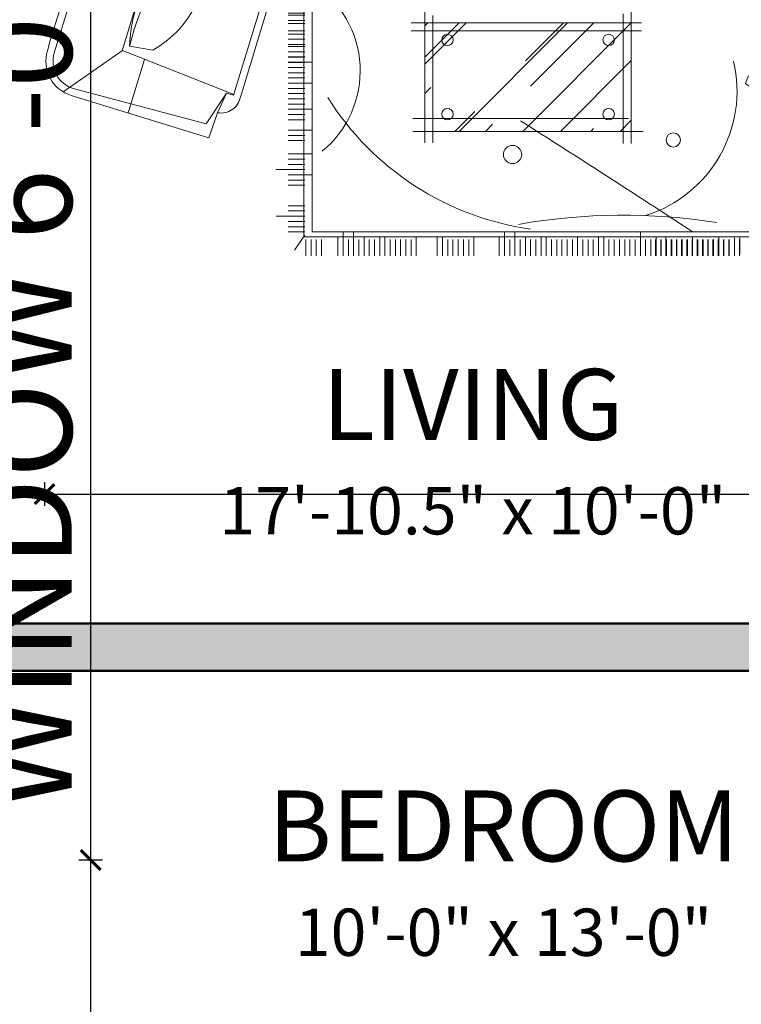
# Model space of a CAD drawing. Units: inches. Extents: x 375 to 1122, y 27 to 1069.
# Tile 73 of 155: x 509 to 601, y 667 to 792. Entities that reach past the tile are written whole.
import ezdxf

# ---------------------------------------------------------------- set-up
doc = ezdxf.new("R2010")
doc.units = ezdxf.units.IN
for name, color, linetype, lineweight in [('A-ANNO-DIMS', 2, 'Continuous', 18), ('A-AREA-IDEN', 7, 'Continuous', 18), ('A-WALL-PATT', 252, 'Continuous', 13), ('Furniture', 30, 'Continuous', 18), ('Walls', 250, 'Continuous', 50)]:
    doc.layers.add(name, color=color, linetype=linetype, lineweight=lineweight)
doc.styles.get("Standard").update_dxf_attribs({"font": 'arial.ttf'})
doc.dimstyles.new('ISO-25', dxfattribs={"dimtxt": 12, "dimasz": 2.5, "dimexe": 1.5, "dimexo": 1.5, "dimtad": 1, "dimdec": 1, "dimlunit": 3, "dimtxsty": 'Standard', "dimblk": 'ARCHTICK', "dimcen": 2.5, "dimadec": 0, "dimazin": 0, "dimtfac": 1, "dimtdec": 1, "dimtmove": 0, "dimatfit": 3, "dimfxl": 1.5, "dimfxlon": 1, "dimarcsym": 0})

# ---------------------------------------------------------------- blocks, each defined once
blk = doc.blocks.new('A$C4DC51D13')
for p, q in [((3265.3, 2996.2), (1188.4, 2996.2)), ((1895.2, 2134), (1895.2, 2996.2)), ((2559.6, 2996.2), (2559.6, 2617.8)), ((277.4, 2939.6), (277.4, 2141.8)), ((943, 2103.5), (943, 2936.7)), ((1188.4, 2962.7), (1862.1, 2962.7)), ((1862.1, 2134), (1862.1, 2962.7)), ((1928.3, 2961.6), (2524.2, 2961.6)), ((1928.3, 2134), (1928.3, 2961.6)), ((2524.2, 2961.6), (2524.2, 2658.6)), ((2590.4, 2962.7), (2590.4, 2654.5)), ((3265.3, 2962.7), (2590.4, 2962.7)), ((1018.2, 2892.3), (232.2, 2892.3)), ((3778.5, 2897), (3631.2, 2747.3)), ((4008.9, 2375.5), (3778.5, 2897)), ((4156.2, 2525.2), (3778.5, 2897)), ((304, 2865.7), (304, 2253.3)), ((916.4, 2865.7), (304, 2865.7)), ((916.4, 2253.3), (916.4, 2865.7)), ((1290.4, 2664.8), (1028, 2870.9)), ((3163.3, 2664.8), (3425.7, 2870.9)), ((1022.9, 2163.8), (1022.9, 2830.3)), ((1056, 2830.3), (1081, 2194.8)), ((3397.7, 2830.3), (3364.5, 2194.8)), ((3430.8, 2163.8), (3430.8, 2830.3)), ((4008.9, 2375.5), (3631.2, 2747.3)), ((423.7, 2370.8), (776.6, 2723.7)), ((427.4, 2727.4), (772.8, 2367.1)), ((497.9, 2644), (497.9, 2699.1)), ((502.2, 2648.3), (502.2, 2701.8)), ((506.4, 2652.2), (506.4, 2704.4)), ((510.6, 2655.8), (510.6, 2706.9)), ((514.9, 2659.2), (514.9, 2709.2)), ((519.1, 2662.3), (519.1, 2711.3)), ((523.3, 2665.1), (523.3, 2713.4)), ((527.5, 2667.8), (527.5, 2715.2)), ((531.8, 2670.2), (531.8, 2717)), ((536, 2672.5), (536, 2718.7)), ((540.2, 2674.6), (540.2, 2720.2)), ((544.4, 2676.5), (544.4, 2721.6)), ((548.7, 2678.2), (548.7, 2722.9)), ((650.1, 2678.8), (650.1, 2723.3)), ((654.3, 2677.1), (654.3, 2722)), ((658.6, 2675.2), (658.6, 2720.7)), ((662.8, 2673.2), (662.8, 2719.2)), ((667, 2671), (667, 2717.6)), ((668.5, 2670.2), (668.5, 2717)), ((671.2, 2668.6), (671.2, 2715.9)), ((672.7, 2667.8), (672.7, 2715.2)), ((675.5, 2666.1), (675.5, 2714)), ((676.9, 2665.1), (676.9, 2713.4)), ((679.7, 2663.3), (679.7, 2712)), ((681.1, 2662.3), (681.1, 2711.3)), ((683.9, 2660.3), (683.9, 2709.9)), ((685.4, 2659.2), (685.4, 2709.2)), ((688.1, 2657), (688.1, 2707.7)), ((689.6, 2655.8), (689.6, 2706.9)), ((692.4, 2653.5), (692.4, 2705.3)), ((693.8, 2652.2), (693.8, 2704.4)), ((696.6, 2649.6), (696.6, 2702.7)), ((698, 2648.3), (698, 2701.8)), ((700.8, 2645.5), (700.8, 2700)), ((702.3, 2644), (702.3, 2699.1)), ((451.5, 2440.6), (451.5, 2654)), ((451.9, 2654.6), (509.2, 2654.6)), ((455.1, 2658.8), (514.4, 2658.8)), ((455.7, 2434.9), (455.7, 2659.6)), ((458.4, 2663.1), (520.2, 2663.1)), ((459.9, 2558.8), (459.9, 2664.9)), ((462, 2667.3), (526.7, 2667.3)), ((464.1, 2583.3), (464.1, 2669.7)), ((465.8, 2671.5), (534.1, 2671.5)), ((468.4, 2596.6), (468.4, 2674.3)), ((469.8, 2675.7), (542.8, 2675.7)), ((472.6, 2606.7), (472.6, 2678.5)), ((476.8, 2615), (476.8, 2682.5)), ((481, 2622.2), (481, 2686.2)), ((485.3, 2628.5), (485.3, 2689.7)), ((489.5, 2634.2), (489.5, 2693)), ((489.5, 2667.3), (489.5, 2633.5)), ((493.7, 2639.3), (493.7, 2696.1)), ((657.4, 2675.7), (730.4, 2675.7)), ((734.5, 2671.5), (666.1, 2671.5)), ((666.1, 2671.5), (734.5, 2671.5)), ((738.2, 2667.3), (673.5, 2667.3)), ((673.5, 2667.3), (738.2, 2667.3)), ((741.8, 2663.1), (680, 2663.1)), ((680, 2663.1), (741.8, 2663.1)), ((745.2, 2658.8), (685.8, 2658.8)), ((685.8, 2658.8), (745.2, 2658.8)), ((748.3, 2654.6), (691, 2654.6)), ((691, 2654.6), (748.3, 2654.6)), ((705, 2641), (705, 2697.2)), ((706.5, 2639.3), (706.5, 2696.1)), ((709.3, 2636), (709.3, 2694.1)), ((710.7, 2634.2), (710.7, 2693)), ((713.5, 2630.5), (713.5, 2690.9)), ((714.9, 2628.5), (714.9, 2689.7)), ((717.7, 2624.4), (717.7, 2687.4)), ((719.2, 2622.2), (719.2, 2686.2)), ((722, 2617.6), (722, 2683.8)), ((723.4, 2615), (723.4, 2682.5)), ((726.2, 2609.7), (726.2, 2679.9)), ((727.6, 2606.7), (727.6, 2678.5)), ((730.4, 2600.3), (730.4, 2675.7)), ((731.9, 2596.6), (731.9, 2674.3)), ((734.6, 2588.4), (734.6, 2671.3)), ((736.1, 2583.3), (736.1, 2669.7)), ((738.9, 2570.4), (738.9, 2666.6)), ((740.3, 2558.8), (740.3, 2664.9)), ((743.1, 2433.1), (743.1, 2661.5)), ((744.5, 2434.9), (744.5, 2659.6)), ((747.3, 2438.6), (747.3, 2656)), ((748.8, 2440.6), (748.8, 2654)), ((1283.3, 2574.2), (1290.4, 2664.8)), ((1290.4, 2664.8), (1894.7, 2664.8)), ((1895.2, 2663.7), (2557.3, 2663.7)), ((2603.6, 2664.8), (2559, 2664.8)), ((3163.3, 2664.8), (2764.7, 2664.8)), ((3170.4, 2574.2), (3163.3, 2664.8)), ((3631.7, 2676.6), (3938.2, 2375)), ((429.1, 2612.3), (475.4, 2612.3)), ((430.3, 2479), (430.3, 2615.5)), ((430.7, 2616.6), (477.7, 2616.6)), ((432.5, 2620.8), (480.2, 2620.8)), ((434.5, 2469.3), (434.5, 2625.2)), ((434.5, 2625), (482.9, 2625)), ((436.5, 2629.2), (485.8, 2629.2)), ((438.7, 2633.5), (488.9, 2633.5)), ((438.8, 2460.9), (438.8, 2633.6)), ((441, 2637.7), (492.3, 2637.7)), ((443, 2453.4), (443, 2641.1)), ((443.5, 2641.9), (496, 2641.9)), ((446.1, 2646.1), (500, 2646.1)), ((447.2, 2446.7), (447.2, 2647.8)), ((448.9, 2650.4), (504.4, 2650.4)), ((751.3, 2650.4), (695.8, 2650.4)), ((695.8, 2650.4), (751.3, 2650.4)), ((754.1, 2646.1), (700.2, 2646.1)), ((700.2, 2646.1), (754.1, 2646.1)), ((756.7, 2641.9), (704.2, 2641.9)), ((704.2, 2641.9), (756.7, 2641.9)), ((759.2, 2637.7), (707.9, 2637.7)), ((707.9, 2637.7), (759.2, 2637.7)), ((761.5, 2633.5), (711.3, 2633.5)), ((711.3, 2633.5), (761.5, 2633.5)), ((763.7, 2629.2), (714.4, 2629.2)), ((714.4, 2629.2), (763.7, 2629.2)), ((765.8, 2625), (717.3, 2625)), ((767.7, 2620.8), (720, 2620.8)), ((769.5, 2616.6), (722.5, 2616.6)), ((771.1, 2612.3), (724.8, 2612.3)), ((751.5, 2444.5), (751.5, 2650)), ((753, 2446.7), (753, 2647.8)), ((755.8, 2451.1), (755.8, 2643.5)), ((757.2, 2453.4), (757.2, 2641.1)), ((760, 2458.3), (760, 2636.3)), ((761.4, 2460.9), (761.4, 2633.6)), ((764.2, 2466.3), (764.2, 2628.2)), ((765.7, 2469.3), (765.7, 2625.2)), ((1798, 2530.2), (1812.1, 2637.9)), ((418.1, 2565.8), (460.7, 2565.8)), ((418.5, 2570.1), (461.3, 2570.1)), ((419.1, 2574.3), (462.1, 2574.3)), ((419.8, 2578.5), (462.9, 2578.5)), ((420.6, 2582.7), (464, 2582.7)), ((421.5, 2587), (465.2, 2587)), ((422.5, 2591.2), (466.5, 2591.2)), ((423.6, 2595.4), (467.9, 2595.4)), ((424.8, 2599.7), (469.6, 2599.7)), ((426.1, 2603.9), (471.3, 2603.9)), ((426.1, 2490.7), (426.1, 2603.9)), ((427.5, 2608.1), (473.3, 2608.1)), ((772.7, 2608.1), (726.9, 2608.1)), ((774.1, 2603.9), (728.9, 2603.9)), ((775.4, 2599.7), (730.7, 2599.7)), ((776.6, 2595.4), (732.3, 2595.4)), ((777.7, 2591.2), (733.7, 2591.2)), ((778.7, 2587), (735.1, 2587)), ((779.6, 2582.7), (736.2, 2582.7)), ((780.4, 2578.5), (737.3, 2578.5)), ((781.1, 2574.3), (738.2, 2574.3)), ((781.7, 2570.1), (738.9, 2570.1)), ((782.2, 2565.8), (739.6, 2565.8)), ((1895.5, 2582.2), (1932.3, 2494.6)), ((417.1, 2548.9), (459.4, 2548.9)), ((417.1, 2544.7), (459.5, 2544.7)), ((417.2, 2553.2), (459.6, 2553.2)), ((417.2, 2540.5), (459.6, 2540.5)), ((417.4, 2557.4), (459.8, 2557.4)), ((417.5, 2536.3), (459.9, 2536.3)), ((417.7, 2561.6), (460.2, 2561.6)), ((417.8, 2532), (460.3, 2532)), ((418.2, 2527.8), (460.8, 2527.8)), ((418.7, 2523.6), (461.4, 2523.6)), ((459.9, 2429.7), (459.9, 2535.7)), ((781.6, 2523.6), (738.8, 2523.6)), ((782.1, 2527.8), (739.4, 2527.8)), ((782.5, 2532), (740, 2532)), ((782.5, 2561.6), (740.1, 2561.6)), ((740.3, 2429.7), (740.3, 2535.7)), ((782.8, 2557.4), (740.4, 2557.4)), ((782.8, 2536.3), (740.4, 2536.3)), ((783, 2540.5), (740.6, 2540.5)), ((783, 2553.2), (740.7, 2553.2)), ((783.1, 2548.9), (740.8, 2548.9)), ((783.1, 2544.7), (740.8, 2544.7)), ((1022.9, 2554.4), (1249.6, 2554.4)), ((2559, 2535.8), (2557.3, 2535.8)), ((3430.8, 2554.4), (3204.1, 2554.4)), ((4008.9, 2375.5), (4156.2, 2525.2)), ((419.3, 2519.4), (462.2, 2519.4)), ((781, 2519.4), (738, 2519.4)), ((1200, 2520.5), (1251.9, 2440.8)), ((3253.7, 2520.5), (3201.8, 2440.8)), ((1243.2, 2146.7), (1272.2, 2431.8)), ((3210.5, 2146.7), (3181.5, 2431.8)), ((242.9, 2226.7), (1018.2, 2226.7)), ((304, 2253.3), (916.4, 2253.3)), ((1081, 2194.8), (1243.2, 2146.7)), ((3364.5, 2194.8), (3210.5, 2146.7)), ((498.8, 1837.1), (382.1, 2139.5)), ((1040.3, 1942.9), (421.2, 2132.6)), ((1145.1, 2159.3), (1022.9, 2163.8)), ((1145.1, 2159.3), (1243.2, 2146.7)), ((1244.8, 2113), (1243.2, 2146.7)), ((2590.4, 2164.3), (2590.4, 2134)), ((3208.9, 2113), (3210.5, 2146.7)), ((3308.6, 2159.3), (3210.5, 2146.7)), ((3308.6, 2159.3), (3430.8, 2163.8)), ((411.8, 2101.9), (992.6, 1890.2)), ((1839.5, 2113), (1244.8, 2113)), ((1839.5, 2079.9), (1244.8, 2079.9)), ((2308.5, 2111.9), (1950.4, 2111.9)), ((2322.1, 2078.8), (1950.4, 2078.8)), ((2614.2, 2113), (3208.9, 2113)), ((2614.2, 2079.9), (3208.9, 2079.9)), ((677.4, 2054.1), (612.9, 1843.6)), ((220.3, 2026), (19.3, 1370.1)), ((251.1, 2016.6), (37.1, 1314.7)), ((1009.7, 1828.1), (1040.3, 1942.9)), ((658.5, 1880), (717.8, 1809.1)), ((992.6, 1890.2), (993.4, 1733.4)), ((1158.3, 1784.3), (1158.3, 1858.2)), ((1181.8, 1784.3), (1181.8, 1858.2)), ((1205.3, 1784.3), (1205.3, 1858.2)), ((1228.8, 1784.3), (1228.8, 1858.2)), ((1252.2, 1784.3), (1252.2, 1858.2)), ((1319.4, 1784.3), (1319.4, 1858.2)), ((1342.9, 1784.3), (1342.9, 1858.2)), ((1366.3, 1784.3), (1366.3, 1858.2)), ((1389.8, 1784.3), (1389.8, 1858.2)), ((1413.3, 1784.3), (1413.3, 1858.2)), ((1436.8, 1784.3), (1436.8, 1858.2)), ((1460.2, 1784.3), (1460.2, 1858.2)), ((1483.7, 1784.3), (1483.7, 1858.2)), ((1507.2, 1784.3), (1507.2, 1858.2)), ((1530.7, 1784.3), (1530.7, 1858.2)), ((1554.1, 1784.3), (1554.1, 1858.2)), ((1577.6, 1784.3), (1577.6, 1858.2)), ((1714.2, 1784.3), (1714.2, 1858.2)), ((1737.6, 1784.3), (1737.6, 1858.2)), ((1761.1, 1784.3), (1761.1, 1858.2)), ((1784.6, 1784.3), (1784.6, 1858.2)), ((1808.1, 1784.3), (1808.1, 1858.2)), ((1831.5, 1784.3), (1831.5, 1858.2)), ((1855, 1784.3), (1855, 1858.2)), ((1878.5, 1784.3), (1878.5, 1858.2)), ((1902, 1784.3), (1902, 1858.2)), ((2050.7, 1784.3), (2050.7, 1858.2)), ((2074.2, 1784.3), (2074.2, 1858.2)), ((2097.7, 1784.3), (2097.7, 1858.2)), ((2121.1, 1784.3), (2121.1, 1858.2)), ((2144.6, 1784.3), (2144.6, 1858.2)), ((2168.1, 1784.3), (2168.1, 1858.2)), ((2238.5, 1785.1), (2238.5, 1859)), ((2262, 1784.3), (2262, 1858.2)), ((2285.4, 1784.3), (2285.4, 1858.2)), ((2543.7, 1784.3), (2543.7, 1858.2)), ((2567.1, 1784.3), (2567.1, 1858.2)), ((2590.6, 1784.3), (2590.6, 1858.2)), ((2614.1, 1784.3), (2614.1, 1858.2)), ((2661, 1784.3), (2661, 1858.2)), ((2684.5, 1784.3), (2684.5, 1858.2)), ((2708, 1772.3), (2708, 1858.2)), ((2731.5, 1784.3), (2731.5, 1858.2)), ((2754.9, 1784.3), (2754.9, 1858.2)), ((2778.4, 1784.3), (2778.4, 1858.2)), ((2801.9, 1784.3), (2801.9, 1858.2)), ((2825.4, 1784.3), (2825.4, 1858.2)), ((2848.8, 1784.3), (2848.8, 1858.2)), ((2872.3, 1784.3), (2872.3, 1858.2)), ((2895.8, 1784.3), (2895.8, 1858.2)), ((2919.3, 1784.3), (2919.3, 1858.2)), ((2942.7, 1784.3), (2942.7, 1858.2)), ((2966.2, 1744.8), (2966.2, 1858.2)), ((2989.7, 1784.3), (2989.7, 1858.2)), ((3013.2, 1772.3), (3013.2, 1858.2)), ((3036.6, 1784.3), (3036.6, 1858.2)), ((3060.1, 1784.3), (3060.1, 1858.2)), ((3083.6, 1784.3), (3083.6, 1858.2)), ((498.8, 1837.1), (341.4, 1323.6)), ((584.9, 1817.9), (498.8, 1837.1)), ((1009.7, 1828.1), (993.4, 1733.4)), ((1158.3, 1821.3), (1158.5, 487.7)), ((2191.6, 1782.4), (2191.6, 1856.3)), ((2215, 1785.7), (2215, 1832.3)), ((993.4, 1733.4), (720.4, 1787.6)), ((1166.1, 1769.7), (1091.8, 1794.5)), ((3248.4, 1772.3), (1158.5, 1772.3)), ((3248.4, 487.7), (3248.4, 1772.3)), ((1024.2, 1722.3), (993.4, 1733.4)), ((1162.1, 1754.9), (1088.2, 1754.9)), ((1162.1, 1741.1), (1088.2, 1741.1)), ((1196, 511), (1196, 1744.8)), ((1196, 1744.8), (3215.6, 1744.8)), ((3215.6, 511), (3215.6, 1744.8)), ((3248.8, 1760.8), (3322.7, 1760.8)), ((3248.8, 1737.3), (3322.7, 1737.3)), ((3600.6, 1621.7), (3605.1, 1743.8)), ((3605.1, 1743.8), (4271.6, 1743.8)), ((3995.7, 1743.8), (3995.7, 1517.1)), ((4106.1, 1476.4), (4312.2, 1738.8)), ((1024.2, 1722.3), (842.3, 1125.2)), ((873.1, 1115.8), (1055, 1712.9)), ((1162.1, 1717.6), (1088.2, 1717.6)), ((1162.1, 1708), (1088.2, 1708)), ((1162.1, 1684.5), (1088.2, 1684.5)), ((3248.8, 1713.8), (3322.7, 1713.8)), ((3248.8, 1690.4), (3322.7, 1690.4)), ((3636.1, 1685.8), (3588, 1523.6)), ((4271.6, 1710.7), (3636.1, 1685.8)), ((3248.8, 1666.9), (3322.7, 1666.9)), ((3248.8, 1643.4), (3322.7, 1643.4)), ((3248.8, 1619.9), (3322.7, 1619.9)), ((3600.6, 1621.7), (3588, 1523.6)), ((4404, 1578.3), (4404, 904.6)), ((4437.5, 165.9), (4437.5, 1578.3)), ((1701.7, 1530), (1701.7, 911.2)), ((3248.8, 1513.8), (3322.7, 1513.8)), ((3248.8, 1513.3), (3322.7, 1513.3)), ((3521.2, 1130.7), (3521.2, 1521.9)), ((3554.3, 1131.4), (3554.3, 1521.9)), ((3588, 1523.6), (3873.1, 1494.5)), ((1162.1, 1492.9), (1088.2, 1492.9)), ((1162.1, 1483.3), (1088.2, 1483.3)), ((1162.1, 1459.8), (1088.2, 1459.8)), ((1737.7, 1483.1), (1737.7, 911.2)), ((2593.1, 907.9), (2593.1, 1490.3)), ((2629.1, 907.9), (2629.1, 1503.1)), ((3248.8, 1490.4), (3322.7, 1490.4)), ((3248.8, 1489.9), (3322.7, 1489.9)), ((3248.8, 1466.9), (3322.7, 1466.9)), ((4015.5, 1483.4), (4106.1, 1476.4)), ((4106.1, 1476.4), (4106.1, 872.1)), ((1162.1, 1446), (1088.2, 1446)), ((2674.6, 1449.9), (1641, 1449.9)), ((1888.1, 1449.9), (1701.7, 1263.5)), ((1856.2, 1449.9), (1701.7, 1295.4)), ((1715.1, 1449.9), (1701.7, 1436.5)), ((2343.3, 1449.9), (1855.3, 961.9)), ((2629.1, 1449), (2142, 961.9)), ((2325.1, 1449.9), (2154.2, 1279.1)), ((2461.6, 1449.9), (2177, 1165.3)), ((3248.8, 1443.4), (3322.7, 1443.4)), ((3248.8, 1419.9), (3322.7, 1419.9)), ((1162.1, 1412.8), (1088.2, 1412.8)), ((1162.1, 1399), (1088.2, 1399)), ((1162.1, 1375.5), (1088.2, 1375.5)), ((2674.6, 1413.9), (1641, 1413.9)), ((3250, 1407.8), (3519, 1407.8)), ((6.3, 1324.2), (19.3, 1370.2)), ((479.3, 1327.3), (375.2, 1344.9)), ((1162.1, 1352.1), (1088.2, 1352.1)), ((1162.1, 1342.9), (1088.2, 1342.9)), ((1162.1, 1342.4), (1088.2, 1342.4)), ((3248.8, 990.8), (3248.4, 1328.4)), ((3248.8, 1359), (3322.7, 1359)), ((342.8, 1324.6), (76.7, 1139.6)), ((843, 1127.6), (342.8, 1324.6)), ((369.2, 1044.8), (442.9, 1285.2)), ((1162.1, 1319.4), (1088.2, 1319.4)), ((1162.1, 1318.9), (1088.2, 1318.9)), ((1162.1, 1296), (1088.2, 1296)), ((1162.1, 1295.5), (1088.2, 1295.5)), ((3248.8, 1312.1), (3322.7, 1312.1)), ((3248.8, 1302.3), (3322.7, 1302.3)), ((3250, 1317.8), (3519, 1317.8)), ((1196, 1272.5), (1088.2, 1272.5)), ((1162.1, 1272), (1088.2, 1272)), ((1162.1, 1249), (1088.2, 1249)), ((1162.1, 1248.5), (1088.2, 1248.5)), ((2629.1, 1280.5), (2310.5, 961.9)), ((3248.8, 1249), (3322.7, 1249)), ((3248.8, 1248.5), (3322.7, 1248.5)), ((3248.8, 1239.3), (3322.7, 1239.3)), ((3248.8, 1238.8), (3322.7, 1238.8)), ((1162.1, 1225.5), (1088.2, 1225.5)), ((1162.1, 1202.1), (1088.2, 1202.1)), ((3248.8, 1225.5), (3322.7, 1225.5)), ((3248.8, 1202.1), (3322.7, 1202.1)), ((122.4, 1154.1), (719.7, 996.3)), ((1196, 1178.6), (1088.2, 1178.6)), ((1162.1, 1155.1), (1088.2, 1155.1)), ((1728.6, 1158.4), (1701.7, 1131.5)), ((3248.8, 1178.6), (3322.7, 1178.6)), ((3248.8, 1155.1), (3322.7, 1155.1)), ((732, 933.5), (112.9, 1123.3)), ((719.7, 996.3), (810.6, 1133.2)), ((771, 1045.7), (810.6, 1133.2)), ((842.3, 1125.2), (810.6, 1133.2)), ((1162.1, 1131.6), (1088.2, 1131.6)), ((1162.1, 1108.2), (1088.2, 1108.2)), ((3248.8, 1131.6), (3322.7, 1131.6)), ((3248.8, 1108.2), (3322.7, 1108.2)), ((1162.1, 1084.7), (1088.2, 1084.7)), ((771, 1045.7), (732, 933.5)), ((1196, 1061.2), (1088.2, 1061.2)), ((1162.1, 1037.7), (1088.2, 1037.7)), ((1648.3, 1019.6), (2616.7, 1019.6)), ((1926.6, 1051.5), (1837.1, 961.9)), ((1162.1, 1014.3), (1088.2, 1014.3)), ((2006.3, 994.6), (1973.6, 961.9)), ((2459.2, 974.1), (2447, 961.9)), ((2629.1, 1012), (2579, 961.9)), ((3248.8, 1014.3), (3322.7, 1014.3)), ((3248.8, 990.8), (3322.7, 990.8)), ((1196, 967.3), (1088.2, 967.3)), ((1162.1, 943.8), (1088.2, 943.8)), ((1648.3, 961.9), (2681.9, 961.9)), ((3248.8, 967.3), (3322.7, 967.3)), ((3248.8, 943.8), (3322.7, 943.8)), ((1162.1, 920.4), (1088.2, 920.4)), ((3248.8, 920.4), (3322.7, 920.4)), ((4097.4, 904.6), (4404, 904.6)), ((1196, 860.5), (1088.2, 860.5)), ((4106.1, 871.5), (4437.5, 871.5)), ((4404, 840.7), (4110.5, 840.7)), ((4404, 165.9), (4404, 840.7)), ((1162.1, 837), (1088.2, 837)), ((1162.1, 813.5), (1088.2, 813.5)), ((3521.2, 816.9), (3521.2, 222.3)), ((3554.3, 816.9), (3554.3, 222.3)), ((1162.1, 790), (1031.8, 790)), ((1196, 766.6), (1088.2, 766.6)), ((1162.1, 743.1), (1088.2, 743.1)), ((1162.1, 719.6), (1088.2, 719.6)), ((4106.1, 267.8), (4106.1, 666.5)), ((1162.1, 627.8), (1088.2, 627.8)), ((3248.8, 627.8), (3322.7, 627.8)), ((1162.1, 580.9), (1034.2, 580.9)), ((1162.1, 604.4), (1088.2, 604.4)), ((3248.8, 604.4), (3322.7, 604.4)), ((3248.8, 580.9), (3322.7, 580.9)), ((1162.1, 557.4), (1088.2, 557.4)), ((1162.1, 533.9), (1088.2, 533.9)), ((3248.8, 557.4), (3322.7, 557.4)), ((3248.8, 533.9), (3322.7, 533.9)), ((1162.1, 510.5), (1088.2, 510.5)), ((1162, 495.1), (1116.6, 429)), ((1158.5, 487.7), (3248.4, 487.7)), ((3215.6, 511), (1196, 511)), ((1311.1, 487.7), (1311.1, 402.4)), ((1334.6, 511), (1334.6, 402.4)), ((1381.6, 511), (1381.6, 402.4)), ((1428.5, 487.7), (1428.5, 402.4)), ((1498.9, 487.7), (1498.9, 402.4)), ((1522.4, 487.7), (1522.4, 402.4)), ((1663.3, 487.7), (1663.3, 402.4)), ((1757.8, 487.7), (1757.8, 402.4)), ((1781.3, 487.7), (1781.3, 402.4)), ((1922.1, 487.7), (1922.1, 402.4)), ((2036, 487.7), (2036, 402.4)), ((2059.5, 511), (2059.5, 402.4)), ((2106.4, 511), (2106.4, 402.4)), ((2153.4, 487.7), (2153.4, 402.4)), ((2223.8, 487.7), (2223.8, 402.4)), ((2247.2, 487.7), (2247.2, 402.4)), ((2388.1, 487.7), (2388.1, 402.4)), ((2482, 487.7), (2482, 402.4)), ((2505.5, 487.7), (2505.5, 402.4)), ((2669.8, 511), (2669.8, 402.4)), ((2740.2, 487.7), (2740.2, 402.4)), ((2784.9, 487.7), (2784.9, 402.4)), ((2904.5, 487.7), (2904.5, 402.4)), ((3021.9, 487.7), (3021.9, 402.4)), ((3244.9, 495.1), (3290.3, 429)), ((3248.8, 510.5), (3322.7, 510.5)), ((1167.1, 476.3), (1167.1, 402.4)), ((1190.6, 476.3), (1190.6, 402.4)), ((1214, 476.3), (1214, 402.4)), ((1237.5, 476.3), (1237.5, 402.4)), ((1358.1, 476.3), (1358.1, 402.4)), ((1405, 476.3), (1405, 402.4)), ((1452, 476.3), (1452, 402.4)), ((1475.5, 476.3), (1475.5, 402.4)), ((1545.9, 476.3), (1545.9, 402.4)), ((1569.4, 476.3), (1569.4, 402.4)), ((1592.8, 476.3), (1592.8, 402.4)), ((1616.3, 476.3), (1616.3, 402.4)), ((1639.8, 476.3), (1639.8, 402.4)), ((1804.8, 476.3), (1804.8, 402.4)), ((1828.2, 476.3), (1828.2, 402.4)), ((1851.7, 476.3), (1851.7, 402.4)), ((1875.2, 476.3), (1875.2, 402.4)), ((1898.7, 476.3), (1898.7, 402.4)), ((2082.9, 476.3), (2082.9, 402.4)), ((2129.9, 476.3), (2129.9, 402.4)), ((2176.8, 476.3), (2176.8, 402.4)), ((2200.3, 476.3), (2200.3, 402.4)), ((2270.7, 476.3), (2270.7, 402.4)), ((2294.2, 476.3), (2294.2, 402.4)), ((2317.7, 476.3), (2317.7, 402.4)), ((2341.1, 476.3), (2341.1, 402.4)), ((2364.6, 476.3), (2364.6, 402.4)), ((2411.6, 476.3), (2411.6, 402.4)), ((2435, 476.3), (2435, 402.4)), ((2458.5, 476.3), (2458.5, 402.4)), ((2528.9, 476.3), (2528.9, 402.4)), ((2552.4, 476.3), (2552.4, 402.4)), ((2575.9, 476.3), (2575.9, 402.4)), ((2599.4, 476.3), (2599.4, 402.4)), ((2622.8, 476.3), (2622.8, 402.4)), ((2646.3, 476.3), (2646.3, 402.4)), ((2693.3, 476.3), (2693.3, 402.4)), ((2716.7, 476.3), (2716.7, 402.4)), ((2738, 476.3), (2738, 402.4)), ((2761.5, 476.3), (2761.5, 402.4)), ((2763.7, 476.3), (2763.7, 402.4)), ((2787.2, 476.3), (2787.2, 402.4)), ((2808.4, 476.3), (2808.4, 402.4)), ((2810.6, 476.3), (2810.6, 402.4)), ((2831.9, 476.3), (2831.9, 402.4)), ((2834.1, 476.3), (2834.1, 402.4)), ((2855.4, 476.3), (2855.4, 402.4)), ((2857.6, 476.3), (2857.6, 402.4)), ((2878.8, 476.3), (2878.8, 402.4)), ((2881.1, 476.3), (2881.1, 402.4)), ((2902.3, 476.3), (2902.3, 402.4)), ((2925.8, 476.3), (2925.8, 402.4)), ((2928, 476.3), (2928, 402.4)), ((2949.3, 476.3), (2949.3, 402.4)), ((2951.5, 476.3), (2951.5, 402.4)), ((2972.7, 476.3), (2972.7, 402.4)), ((2975, 476.3), (2975, 402.4)), ((2996.2, 476.3), (2996.2, 402.4)), ((2998.4, 476.3), (2998.4, 402.4)), ((3019.7, 476.3), (3019.7, 402.4)), ((3043.2, 476.3), (3043.2, 402.4)), ((3045.4, 476.3), (3045.4, 402.4)), ((3066.6, 476.3), (3066.6, 402.4)), ((3068.9, 476.3), (3068.9, 402.4)), ((3092.3, 476.3), (3092.3, 402.4)), ((3092.7, 484.5), (3092.7, 410.6)), ((3115.8, 476.3), (3115.8, 402.4)), ((3116.2, 484.5), (3116.2, 410.6)), ((3202.2, 476.3), (3202.2, 402.4)), ((3225.7, 476.3), (3225.7, 402.4)), ((3249.2, 476.3), (3249.2, 402.4)), ((4015.5, 260.8), (4106.1, 267.8)), ((4106.1, 267.8), (4312.2, 5.4)), ((3588, 220.6), (3873.1, 249.7)), ((3961.8, 177.4), (3882.1, 229.3)), ((3995.7, 0.4), (3995.7, 227)), ((3636.1, 66.6), (3588, 220.6)), ((3600.6, 122.5), (3605.1, 0.4)), ((4271.6, 33.5), (3636.1, 66.6)), ((3605.1, 0.4), (4271.6, 0.4))]:
    blk.add_line(p, q)
at = {"linetype": 'ByBlock'}
for points in [[(2342.9, 1843.9), (2352.5, 1810.4), (2340.1, 1777.7), (2351.8, 1757), (2412.3, 1818), (2433.1, 1866.4), (2453.1, 1889.5), (2436, 1914.7), (2407.6, 1926.2), (2433.7, 1959.9), (2473.1, 2048.3), (2530.6, 2101.1), (2625.9, 2180.3), (2669, 2174.2), (2748.1, 2315.4), (2745.8, 2342.6), (2801.2, 2404.9), (2823.9, 2479.6), (2818.4, 2529.9), (2775.1, 2571.7), (2782.4, 2583.3), (2765.2, 2658.8), (2714.5, 2706.9), (2634.6, 2708.6), (2571.9, 2652.6), (2548.8, 2649.4), (2474, 2672.1), (2312.9, 2542.1), (2312.9, 2341.6), (2333.9, 2336.4), (2302, 2223.9), (2313.6, 2216.6), (2297.4, 2095.7), (2309.3, 2034.9), (2320.2, 1952), (2319.3, 1929.9), (2280.8, 1863.6), (2257.7, 1842.4), (2239.2, 1825.7), (2220.1, 1798.2), (2221.6, 1713.1), (2254.3, 1700.7), (2275.9, 1729.8), (2288.6, 1768), (2313.7, 1797.6)], [(3285.2, 1088.3), (3251.7, 1078.6), (3219, 1091.1), (3198.3, 1079.4), (3259.3, 1018.8), (3307.7, 998), (3330.8, 978), (3356, 995.1), (3367.5, 1023.6), (3401.2, 997.5), (3489.6, 958), (3542.4, 900.5), (3621.6, 805.3), (3615.5, 762.2), (3756.7, 683), (3783.9, 685.3), (3846.2, 629.9), (3920.9, 607.2), (3971.2, 612.7), (4013, 656), (4024.6, 648.7), (4100.1, 665.9), (4148.2, 716.6), (4149.9, 796.5), (4093.9, 859.3), (4090.7, 882.4), (4113.4, 957.1), (3983.4, 1118.2), (3782.9, 1118.2), (3777.7, 1097.2), (3665.2, 1129.2), (3657.9, 1117.6), (3537, 1133.7), (3476.2, 1121.9), (3393.3, 1110.9), (3371.2, 1111.9), (3304.9, 1150.4), (3283.7, 1173.4), (3267, 1191.9), (3239.5, 1211), (3154.4, 1209.5), (3142, 1176.8), (3171.1, 1155.3), (3209.3, 1142.5), (3238.9, 1117.5)]]:
    blk.add_lwpolyline(points, close=True, dxfattribs=at)
for points in [[(2563.4, 2654.7), (2512.2, 2609.3), (2506.2, 2548.3), (2540.1, 2504.4), (2576.9, 2490.9), (2579.8, 2539.3), (2598.7, 2543.6), (2636.7, 2516.4), (2690.3, 2516.7), (2731.2, 2520.1), (2758.5, 2540.1), (2773, 2563.3)], [(2629.1, 2357.8), (2507, 2405.5), (2433.2, 2450.3), (2445.5, 2500.8), (2478.9, 2546.1), (2402.4, 2506.9), (2373.4, 2424.8), (2384.4, 2341.9), (2352.8, 2340.7)], [(2712.3, 2515.8), (2652.7, 2472.4), (2603.2, 2489), (2580, 2503.6)], [(2738, 2438.2), (2699.2, 2425.4), (2742.4, 2401.4), (2680.4, 2403.2), (2604.1, 2328.3), (2519.2, 2273.3), (2529.8, 2261.8), (2402.7, 2252.7), (2395.4, 2241.1), (2431.1, 2241.3), (2375.7, 2196.9), (2385.2, 2181.2), (2474.4, 2199.5), (2549.9, 2234.6), (2596.2, 2223.2), (2730.1, 2333.1)], [(2433.2, 2450.3), (2377.6, 2423.8)], [(2409.5, 2153), (2387.5, 2153.9), (2359, 2165.4), (2352.6, 2193.7), (2353.5, 2215.7), (2330.5, 2194.6), (2322.1, 2196.7), (2341.8, 2240.9), (2345.5, 2329.1)], [(2374.9, 2339.8), (2395.2, 2276.9)], [(2613.2, 2183.4), (2541.6, 2218.8)], [(2431.4, 2187.8), (2379.5, 2066.7), (2320.2, 1929.7)], [(2407.6, 1926.2), (2342.9, 1843.9)], [(2412.9, 1911.5), (2401.6, 1865.2), (2361.9, 1812.5)], [(2279.2, 1765.9), (2259.2, 1757.4), (2247.6, 1764.7), (2246.4, 1796.2), (2253.5, 1843.5)], [(3207.2, 1152), (3198.7, 1171.9), (3206, 1183.5), (3237.5, 1184.7), (3284.8, 1177.6)], [(3629.1, 999.7), (3508, 1051.6), (3371, 1110.9)], [(3594.3, 1021.6), (3595.2, 1043.7), (3606.7, 1072.1), (3635, 1078.6), (3657, 1077.6), (3635.9, 1100.6), (3638, 1109.1), (3682.2, 1089.3), (3770.4, 1085.6)], [(3352.8, 1018.2), (3306.5, 1029.5), (3253.8, 1069.2)], [(3367.5, 1023.6), (3285.2, 1088.3)], [(3799.1, 802), (3846.8, 924.2), (3891.6, 998), (3942.1, 985.6), (3987.4, 952.2), (3948.2, 1028.7), (3866.1, 1057.7), (3783.2, 1046.8), (3782, 1078.3)], [(3879.5, 693.2), (3866.7, 732), (3842.7, 688.8), (3844.5, 750.8), (3769.6, 827.1), (3714.6, 911.9), (3703.1, 901.3), (3694, 1028.4), (3682.4, 1035.7), (3682.6, 1000), (3638.2, 1055.5), (3622.5, 1045.9), (3640.8, 956.7), (3675.9, 881.2), (3664.5, 834.9), (3774.4, 701)], [(3781.1, 1056.2), (3718.2, 1035.9)], [(3891.6, 998), (3865.1, 1053.5)], [(3624.7, 817.9), (3660.1, 889.6)], [(4096, 867.7), (4050.6, 918.9), (3989.6, 924.9), (3945.7, 891.1), (3932.2, 854.2), (3980.6, 851.3), (3984.9, 832.4), (3957.7, 794.4), (3958, 740.9), (3961.4, 699.9), (3981.4, 672.7), (4004.6, 658.1)], [(3957.1, 718.8), (3913.7, 778.5), (3930.3, 827.9), (3944.9, 851.1)]]:
    blk.add_lwpolyline(points, dxfattribs=at)
for centre, radius in [((600.1, 2547.3), 183), ((600.1, 2547.3), 140.7), ((1803.2, 1372.6), 25.7), ((2527.6, 1372.6), 25.7), ((1803.2, 1039.3), 25.7), ((2527.6, 1039.3), 25.7), ((2817.9, 923.4), 31.7), ((2095.7, 858), 41)]:
    blk.add_circle(centre, radius)
for centre, radius, start, end in [((1188.4, 2830.3), 165.9, 90, 180), ((3265.3, 2830.3), 165.9, 0, 90), ((1188.4, 2830.3), 132.4, 90, 180), ((3265.3, 2830.3), 132.4, 0, 90), ((3666.8, 2712.2), 50, 135.4503, 225.4503), ((1626.8, 1949.8), 712.7, 74.928, 126.7929), ((2192.2, 2032.6), 624.6, 69.4145, 118.3621), ((2633.9, 373.6), 2292.5, 91.8726, 91.9144), ((2832.8, 1963.1), 698.5, 52.9389, 95.0789), ((1707.9, 1527), 1115.8, 84.6406, 117.0804), ((2210.2, 1780.8), 852.5, 76.866, 111.6839), ((2713.3, 1357.7), 1282.3, 65.0725, 87.2152), ((1459.9, 2882.7), 488.4, 244.7866, 313.8058), ((2216, 2892.1), 488.4, 234.4888, 282.1285), ((2993.8, 2882.7), 488.4, 248.2152, 295.2134), ((3973.2, 2410.6), 50, 225.4503, 315.4503), ((374.1, 1978.9), 160.8, 72.9571, 162.9571), ((1234.5, 2169.3), 90, 186.4251, 276.5821), ((1839.5, 2135.1), 22.1, 270, 0), ((1839.5, 2135.1), 55.2, 270, 0), ((1950.4, 2134), 55.2, 180, 270), ((1950.4, 2134), 22.1, 180, 270), ((2619.6, 2148.3), 68.5, 191.0595, 265.4426), ((2614.2, 2135.1), 22.1, 180, 270), ((3219.2, 2169.3), 90, 263.4179, 353.5749), ((374.1, 1978.9), 128.6, 72.9571, 162.9571), ((1584.7, 1047), 1245.7, 138.0296, 166.1636), ((1067.1, 1321), 692.3, 126.1642, 178.0291), ((974.8, 1747.9), 87.4, 336.375, 66.532), ((248.2, 1741.7), 474.4, 299.1514, 8.1705), ((4271.6, 1578.3), 165.9, 0, 90), ((4271.6, 1578.3), 132.4, 0, 90), ((944.2, 1233.8), 467.1, 309.4804, 56.621), ((3610.6, 1532.2), 90, 96.4251, 186.5821), ((3383, 1136.2), 721.4, 348.1046, 36.6442), ((2968.3, 1058.8), 1115.8, 356.7543, 27.0804), ((4324, 1306.8), 488.4, 154.7866, 202.7137), ((160.1, 1277), 160.8, 162.9571, 252.9571), ((160.1, 1277), 128.6, 162.9571, 252.9571), ((2517.5, 1143.6), 586.7, 287.3395, 13.1463), ((787.1, 1131.7), 87.4, 259.3822, 349.5393), ((2356.9, 1798.1), 1287.8, 212.1153, 261.9323), ((-29968.2, -49615.7), 59944, 56.743614, 57.623407), ((3404.4, 598.4), 698.5, 322.9389, 5.0789), ((2799, 717.9), 1282.3, 335.0725, 357.2152), ((2591.9, -2109.1), 2694.5, 80.9842, 100.0261), ((4324, 437.4), 488.4, 158.2152, 205.2134), ((3610.6, 212), 90, 173.4179, 263.5749), ((4271.6, 165.9), 132.4, 270, 0), ((4271.6, 165.9), 165.9, 270, 0)]:
    blk.add_arc(centre, radius, start, end)
blk = doc.blocks.new('_ArchTick')
at = {"color": 0, "linetype": 'ByBlock', "const_width": 0.15}
blk.add_lwpolyline([(-0.5, -0.5), (0.5, 0.5)], dxfattribs=at)
blk = doc.blocks.new('*D43')
at = {"layer": 'A-ANNO-DIMS', "color": 0, "lineweight": -2, "transparency": 16777216}
for p, q in [((617.28, 580.53), (617.28, 790.11)), ((615.78, 580.53), (618.78, 580.53)), ((617.28, 513.06), (617.28, 580.53)), ((615.78, 513.06), (618.78, 513.06))]:
    blk.add_line(p, q, dxfattribs=at)
at = {"layer": 'Defpoints', "color": 0, "transparency": 16777216}
for p in [(607.16, 580.53), (617.28, 580.53), (607.16, 513.06)]:
    blk.add_point(p, dxfattribs=at)
at = {"layer": 'A-ANNO-DIMS', "color": 0, "lineweight": -2, "transparency": 16777216, "xscale": 2.5, "yscale": 2.5, "zscale": 2.5}
for p, rotation in [((617.28, 580.53), 90), ((617.28, 513.06), 270)]:
    blk.add_blockref('_ArchTick', p, dxfattribs=dict(at, rotation=rotation))
at = {"layer": 'A-ANNO-DIMS', "color": 0, "transparency": 16777216, "insert": (610.45, 686.57), "char_height": 12, "attachment_point": 5, "rotation": 90}
blk.add_mtext('BED GROUP 5\'-7 1/2" TYP.', dxfattribs=at)
blk = doc.blocks.new('*D45')
at = {"layer": 'A-ANNO-DIMS', "color": 0, "lineweight": -2, "transparency": 16777216}
for p, q in [((697.69, 641.67), (697.69, 644.67)), ((722.01, 641.67), (722.01, 644.67)), ((697.69, 643.17), (559.76, 643.17)), ((722.01, 643.17), (697.69, 643.17))]:
    blk.add_line(p, q, dxfattribs=at)
at = {"layer": 'Defpoints', "color": 0, "transparency": 16777216}
for p in [(697.69, 643.17), (697.69, 639.53), (722.01, 639.53)]:
    blk.add_point(p, dxfattribs=at)
at = {"layer": 'A-ANNO-DIMS', "color": 0, "lineweight": -2, "transparency": 16777216, "xscale": 2.5, "yscale": 2.5, "zscale": 2.5, "rotation": 180}
blk.add_blockref('_ArchTick', (697.69, 643.17), dxfattribs=at)
at = {"layer": 'A-ANNO-DIMS', "color": 0, "lineweight": -2, "transparency": 16777216, "xscale": 2.5, "yscale": 2.5, "zscale": 2.5}
blk.add_blockref('_ArchTick', (722.01, 643.17), dxfattribs=at)
at = {"layer": 'A-ANNO-DIMS', "color": 0, "transparency": 16777216, "insert": (627.47, 650), "char_height": 12, "attachment_point": 5}
blk.add_mtext('WC 2\'-0 1/2" TYP.', dxfattribs=at)
blk = doc.blocks.new('*D57')
at = {"layer": 'A-ANNO-DIMS', "color": 0, "lineweight": -2, "transparency": 16777216}
for p, q in [((512.46, 733.49), (512.46, 730.49)), ((638.07, 733.49), (638.07, 730.49)), ((512.46, 731.99), (638.07, 731.99)), ((638.07, 731.99), (839.76, 731.99))]:
    blk.add_line(p, q, dxfattribs=at)
at = {"layer": 'Defpoints', "color": 0, "transparency": 16777216}
for p in [(512.46, 750.84), (638.07, 750.84), (638.07, 731.99)]:
    blk.add_point(p, dxfattribs=at)
at = {"layer": 'A-ANNO-DIMS', "color": 0, "lineweight": -2, "transparency": 16777216, "xscale": 2.5, "yscale": 2.5, "zscale": 2.5, "rotation": 180}
blk.add_blockref('_ArchTick', (512.46, 731.99), dxfattribs=at)
at = {"layer": 'A-ANNO-DIMS', "color": 0, "lineweight": -2, "transparency": 16777216, "xscale": 2.5, "yscale": 2.5, "zscale": 2.5}
blk.add_blockref('_ArchTick', (638.07, 731.99), dxfattribs=at)
at = {"layer": 'A-ANNO-DIMS', "color": 0, "transparency": 16777216, "insert": (740.16, 738.83), "char_height": 12, "attachment_point": 5}
blk.add_mtext('SOFA SET 10\'-5 1/2" TYP.', dxfattribs=at)
blk = doc.blocks.new('*D69')
at = {"layer": 'A-ANNO-DIMS', "color": 0, "lineweight": -2, "transparency": 16777216}
for p, q in [((518.31, 685.53), (518.31, 841.13)), ((516.81, 685.53), (519.81, 685.53)), ((518.31, 613.53), (518.31, 685.53)), ((516.81, 613.53), (519.81, 613.53))]:
    blk.add_line(p, q, dxfattribs=at)
at = {"layer": 'Defpoints', "color": 0, "transparency": 16777216}
for p in [(507.51, 685.53), (518.31, 685.53), (507.51, 613.53)]:
    blk.add_point(p, dxfattribs=at)
at = {"layer": 'A-ANNO-DIMS', "color": 0, "lineweight": -2, "transparency": 16777216, "xscale": 2.5, "yscale": 2.5, "zscale": 2.5}
for p, rotation in [((518.31, 685.53), 90), ((518.31, 613.53), 270)]:
    blk.add_blockref('_ArchTick', p, dxfattribs=dict(at, rotation=rotation))
at = {"layer": 'A-ANNO-DIMS', "color": 0, "transparency": 16777216, "insert": (511.47, 764.58), "char_height": 12, "attachment_point": 5, "rotation": 90}
blk.add_mtext('WINDOW 6\'-0" TYP.', dxfattribs=at)
blk = doc.blocks.new('*D82')
at = {"layer": 'A-ANNO-DIMS', "color": 0, "lineweight": -2, "transparency": 16777216}
for p, q in [((401.51, 1009.53), (398.51, 1009.53)), ((400.01, 160.53), (400.01, 1009.53)), ((401.51, 160.53), (398.51, 160.53))]:
    blk.add_line(p, q, dxfattribs=at)
at = {"layer": 'Defpoints', "color": 0, "transparency": 16777216}
for p in [(400.01, 1009.53), (630.53, 1009.53), (630.53, 160.53)]:
    blk.add_point(p, dxfattribs=at)
at = {"layer": 'A-ANNO-DIMS', "color": 0, "lineweight": -2, "transparency": 16777216, "xscale": 2.5, "yscale": 2.5, "zscale": 2.5}
for p, rotation in [((400.01, 1009.53), 90), ((400.01, 160.53), 270)]:
    blk.add_blockref('_ArchTick', p, dxfattribs=dict(at, rotation=rotation))
at = {"layer": 'A-ANNO-DIMS', "color": 0, "transparency": 16777216, "insert": (393.26, 585.03), "char_height": 12, "attachment_point": 5, "rotation": 90}
blk.add_mtext('70\'-9"', dxfattribs=at)
blk = doc.blocks.new('*D93')
at = {"layer": 'A-ANNO-DIMS', "color": 0, "lineweight": -2, "transparency": 16777216}
for p, q in [((400.01, 673.53), (400.01, 709.38)), ((401.51, 673.53), (398.51, 673.53)), ((400.01, 649.53), (400.01, 673.53)), ((401.51, 649.53), (398.51, 649.53))]:
    blk.add_line(p, q, dxfattribs=at)
at = {"layer": 'Defpoints', "color": 0, "transparency": 16777216}
for p in [(400.01, 673.53), (663.51, 673.53), (663.51, 649.53)]:
    blk.add_point(p, dxfattribs=at)
at = {"layer": 'A-ANNO-DIMS', "color": 0, "lineweight": -2, "transparency": 16777216, "xscale": 2.5, "yscale": 2.5, "zscale": 2.5}
for p, rotation in [((400.01, 673.53), 90), ((400.01, 649.53), 270)]:
    blk.add_blockref('_ArchTick', p, dxfattribs=dict(at, rotation=rotation))
at = {"layer": 'A-ANNO-DIMS', "color": 0, "transparency": 16777216, "insert": (393.26, 692.7), "char_height": 12, "attachment_point": 5, "rotation": 90}
blk.add_mtext('2\'-0"', dxfattribs=at)

msp = doc.modelspace()

# ---------------------------------------------------------------- hatches: boundary and pattern name
at = {"layer": 'A-WALL-PATT'}
h = msp.add_hatch(color=256, dxfattribs=at)
h.dxf.hatch_style = 1
h.paths.add_polyline_path([(962.01, 388.53), (989.01, 388.53), (989.01, 394.53), (962.01, 394.53), (932.01, 394.53), (932.01, 397.53), (923.01, 397.53), (923.01, 394.53), (842.01, 394.53), (842.01, 334.53), (839.51, 334.53), (839.51, 328.53), (854.01, 328.53), (854.01, 334.53), (848.01, 334.53), (848.01, 388.53), (953.01, 388.53), (953.01, 356.08), (962.01, 356.08), (962.01, 358.55), (989.01, 358.55), (989.01, 364.55), (962.01, 364.55)])
h.paths.add_polyline_path([(989.01, 502.53), (932.01, 502.53), (932.01, 583.53), (932.01, 593.53), (923.01, 593.53), (923.01, 583.53), (854.01, 583.53), (854.01, 556.53), (863.01, 556.53), (863.01, 574.53), (923.01, 574.53), (923.01, 502.53), (863.01, 502.53), (863.01, 520.53), (854.01, 520.53), (854.01, 502.53), (773.01, 502.53), (773.01, 493.53), (788.01, 493.53), (788.01, 402.03), (722.01, 402.03), (722.01, 373.53), (728.01, 373.53), (728.01, 396.03), (788.01, 396.03), (788.01, 373.53), (794.01, 373.53), (794.01, 430.53), (814.01, 430.53), (814.01, 436.53), (794.01, 436.53), (794.01, 493.53), (923.01, 493.53), (923.01, 487.53), (932.01, 487.53), (932.01, 493.53), (983.01, 493.53), (983.01, 473.53), (989.01, 473.53)])
h.paths.add_polyline_path([(797.01, 325.53), (805.01, 325.53), (805.01, 328.53), (807.51, 328.53), (807.51, 334.53), (791.01, 334.53), (791.01, 226.53), (770.76, 226.53), (770.76, 217.53), (791.01, 217.53), (791.01, 187.53), (855.01, 187.53), (855.01, 196.53), (797.01, 196.53)])
h.paths.add_polyline_path([(989.01, 238.53), (962.01, 238.53), (962.01, 256.42), (953.01, 256.42), (953.01, 229.53), (980.01, 229.53), (980.01, 196.53), (915.01, 196.53), (915.01, 187.53), (989.01, 187.53)])
h.paths.add_polyline_path([(962.01, 334.53), (884.01, 334.53), (884.01, 328.53), (918.01, 328.53), (918.01, 325.53), (932.01, 325.53), (932.01, 328.53), (953.01, 328.53), (953.01, 304.42), (962.01, 304.42)])
h.paths.add_polyline_path([(606.51, 283.53), (609.51, 283.53), (609.51, 289.53), (600.51, 289.53), (600.51, 196.53), (578.51, 196.53), (578.51, 187.53), (606.51, 187.53), (606.51, 196.53)])
h.paths.add_polyline_path([(666.51, 292.53), (660.51, 292.53), (660.51, 289.53), (633.51, 289.53), (633.51, 283.53), (660.51, 283.53), (660.51, 196.53), (628.01, 196.53), (628.01, 187.53), (630.53, 187.53), (630.53, 160.53), (636.53, 160.53), (636.53, 187.53), (660.51, 187.53), (660.51, 160.53), (666.51, 160.53), (666.51, 217.53), (686.76, 217.53), (686.76, 226.53), (666.51, 226.53)])
h.paths.add_polyline_path([(480.51, 256.42), (471.51, 256.42), (471.51, 238.53), (444.51, 238.53), (444.51, 187.53), (518.51, 187.53), (518.51, 196.53), (453.51, 196.53), (453.51, 229.53), (480.51, 229.53)])
h.paths.add_polyline_path([(480.51, 328.53), (652.51, 328.53), (652.51, 325.53), (660.51, 325.53), (660.51, 322.53), (666.51, 322.53), (666.51, 334.53), (507.51, 334.53), (507.51, 360.53), (498.51, 360.53), (498.51, 334.53), (471.51, 334.53), (471.51, 304.42), (480.51, 304.42)])
h.paths.add_polyline_path([(507.51, 484.53), (498.51, 484.53), (498.51, 444.53), (507.51, 444.53), (507.51, 454.53), (621.51, 454.53), (621.51, 460.53), (507.51, 460.53)])
h.paths.add_polyline_path([(672.51, 604.53), (683.26, 604.53), (683.26, 613.53), (669.51, 613.53), (669.51, 649.53), (663.51, 649.53), (663.51, 589.53), (507.51, 589.53), (507.51, 613.53), (498.51, 613.53), (498.51, 556.53), (507.51, 556.53), (507.51, 580.53), (663.51, 580.53), (663.51, 520.53), (669.51, 520.53), (669.51, 556.53), (683.26, 556.53), (683.26, 565.53), (672.51, 565.53)])
h.paths.add_polyline_path([(731.01, 667.53), (734.01, 667.53), (734.01, 676.53), (728.01, 676.53), (728.01, 715.53), (657.51, 715.53), (657.51, 709.53), (663.51, 709.53), (663.51, 673.53), (669.51, 673.53), (669.51, 709.53), (722.01, 709.53), (722.01, 613.53), (704.76, 613.53), (704.76, 604.53), (722.01, 604.53), (722.01, 565.53), (704.76, 565.53), (704.76, 556.53), (722.01, 556.53), (722.01, 502.53), (722.01, 460.53), (669.51, 460.53), (669.51, 496.53), (663.51, 496.53), (663.51, 460.53), (657.51, 460.53), (657.51, 454.53), (728.01, 454.53), (728.01, 493.53), (734.01, 493.53), (734.01, 502.53), (731.01, 502.53)])
h.paths.add_polyline_path([(986.01, 718.53), (959.01, 718.53), (959.01, 727.53), (950.01, 727.53), (950.01, 709.53), (977.01, 709.53), (977.01, 676.53), (794.01, 676.53), (794.01, 805.53), (802.01, 805.53), (802.01, 808.53), (804.51, 808.53), (804.51, 814.53), (788.01, 814.53), (788.01, 774.03), (728.01, 774.03), (728.01, 796.53), (722.01, 796.53), (722.01, 768.03), (788.01, 768.03), (788.01, 676.53), (773.01, 676.53), (773.01, 667.53), (923.01, 667.53), (923.01, 657.53), (932.01, 657.53), (932.01, 667.53), (986.01, 667.53)])
h.paths.add_polyline_path([(621.51, 715.53), (507.51, 715.53), (507.51, 733.53), (498.51, 733.53), (498.51, 715.53), (498.51, 685.53), (507.51, 685.53), (507.51, 709.53), (621.51, 709.53)])
h.paths.add_polyline_path([(666.51, 847.03), (660.51, 847.03), (660.51, 844.53), (652.51, 844.53), (652.51, 841.53), (480.51, 841.53), (480.51, 859.53), (471.51, 859.53), (471.51, 835.53), (498.51, 835.53), (498.51, 817.53), (507.51, 817.53), (507.51, 835.53), (666.51, 835.53)])
h.paths.add_polyline_path([(480.51, 940.53), (453.51, 940.53), (453.51, 973.53), (518.51, 973.53), (518.51, 982.53), (444.51, 982.53), (444.51, 931.53), (471.51, 931.53), (471.51, 907.53), (480.51, 907.53)])
h.paths.add_polyline_path([(606.51, 982.53), (578.51, 982.53), (578.51, 973.53), (600.51, 973.53), (600.51, 880.53), (609.51, 880.53), (609.51, 886.53), (606.51, 886.53)])
h.paths.add_polyline_path([(666.51, 943.53), (686.76, 943.53), (686.76, 952.53), (666.51, 952.53), (666.51, 1009.53), (660.51, 1009.53), (660.51, 982.53), (636.53, 982.53), (636.53, 1009.53), (630.53, 1009.53), (630.53, 982.53), (628.01, 982.53), (628.01, 973.53), (660.51, 973.53), (660.51, 886.53), (633.51, 886.53), (633.51, 880.53), (660.51, 880.53), (660.51, 877.03), (666.51, 877.03)])
h.paths.add_polyline_path([(986.01, 874.53), (932.01, 874.53), (932.01, 877.53), (923.01, 877.53), (923.01, 874.53), (788.01, 874.53), (788.01, 868.53), (788.01, 844.53), (794.01, 844.53), (794.01, 868.53), (839.01, 868.53), (839.01, 814.53), (836.51, 814.53), (836.51, 808.53), (851.01, 808.53), (851.01, 814.53), (845.01, 814.53), (845.01, 868.53), (986.01, 868.53)])
h.paths.add_polyline_path([(959.01, 838.55), (986.01, 838.55), (986.01, 844.55), (959.01, 844.55), (959.01, 847.03), (950.01, 847.03), (950.01, 814.53), (881.01, 814.53), (881.01, 808.53), (918.01, 808.53), (918.01, 805.53), (932.01, 805.53), (932.01, 808.53), (950.01, 808.53), (950.01, 793.53), (959.01, 793.53)])
h.paths.add_polyline_path([(986.01, 982.53), (899.01, 982.53), (899.01, 973.53), (923.01, 973.53), (923.01, 967.53), (932.01, 967.53), (932.01, 973.53), (980.01, 973.53), (980.01, 953.53), (986.01, 953.53)])
h.paths.add_polyline_path([(851.01, 982.53), (788.01, 982.53), (788.01, 952.53), (770.76, 952.53), (770.76, 943.53), (788.01, 943.53), (788.01, 910.53), (814.01, 910.53), (814.01, 916.53), (794.01, 916.53), (794.01, 973.53), (851.01, 973.53)])

# ---------------------------------------------------------------- linework, layer by layer
at = {"layer": 'Walls'}
for p, q in [((507.51, 715.53), (621.51, 715.53)), ((507.51, 709.53), (621.51, 709.53))]:
    msp.add_line(p, q, dxfattribs=at)

# ---------------------------------------------------------------- block references
at = {"layer": 'Furniture', "xscale": 0.0282665567793757, "yscale": 0.0282665567793757, "zscale": 0.0282665567793757}
msp.add_blockref('A$C4DC51D13', (512.64, 750.84), dxfattribs=at)

# ---------------------------------------------------------------- texts
at = {"layer": 'A-AREA-IDEN', "char_height": 12, "attachment_point": 7}
for s, width, insert in [('\\pxqc;{\\fArial|b1|i0|c0|p34;\\H0.75x;LIVING\\H1.33333x;\\P\\fArial|b0|i0|c0|p34;\\H0.5x;17\'-10.5" x 10\'-0"}', 66.1169, (533.78, 726.86)), ('\\pxqc;{\\fArial|b1|i0|c0|p34;\\H0.75x;BEDROOM\\H1.33333x;\\P\\fArial|b0|i0|c0|p34;\\H0.5x;10\'-0" x 13\'-0"}', 73.8986, (533.78, 673.35))]:
    msp.add_mtext_dynamic_manual_height_columns(s, width=width, gutter_width=12.5, heights=[0], dxfattribs=dict(at, insert=insert))

# ---------------------------------------------------------------- dimensions: what is measured, and where the dimension line sits
at = {"layer": 'A-ANNO-DIMS'}
for base, p1, p2, picture, middle in [((400.01, 1009.53), (630.53, 160.53), (630.53, 1009.53), '*D82', (393.26, 585.03)), ((400.01, 673.53), (663.51, 649.53), (663.51, 673.53), '*D93', (393.26, 692.7))]:
    dim = msp.add_linear_dim(base=base, p1=p1, p2=p2, angle=90, dimstyle='ISO-25', override={"dimdec": 1, "dimlfac": 1, "dimrnd": 0, "dimzin": 1, "dimdsep": 46, "dimlunit": 4, "dimfrac": 2}, dxfattribs=at)
    dim.commit()
    dim.dimension.update_dxf_attribs({"geometry": picture, "text_midpoint": middle})
for base, p1, p2, angle, text, picture, middle in [((518.31, 685.53), (507.51, 613.53), (507.51, 685.53), 90, 'WINDOW <> TYP.', '*D69', (511.47, 764.58)), ((617.28, 580.53), (607.16, 513.06), (607.16, 580.53), 90, 'BED GROUP <> TYP.', '*D43', (610.45, 686.57)), ((697.69, 643.17), (722.01, 639.53), (697.69, 639.53), 180, 'WC <> TYP.', '*D45', (627.47, 650))]:
    dim = msp.add_linear_dim(base=base, p1=p1, p2=p2, angle=angle, text=text, dimstyle='ISO-25', override={"dimdec": 1, "dimlfac": 1, "dimrnd": 0, "dimzin": 1, "dimdsep": 46, "dimlunit": 4, "dimfrac": 2}, dxfattribs=at)
    dim.commit()
    dim.dimension.update_dxf_attribs({"geometry": picture, "text_midpoint": middle})
dim = msp.add_linear_dim(base=(638.07, 731.99), p1=(512.46, 750.84), p2=(638.07, 750.84), text='SOFA SET <> TYP.', dimstyle='ISO-25', override={"dimdec": 1, "dimlfac": 1, "dimrnd": 0, "dimzin": 1, "dimdsep": 46, "dimlunit": 4, "dimfrac": 2}, dxfattribs=at)
dim.commit()
dim.dimension.update_dxf_attribs({"geometry": '*D57', "text_midpoint": (740.16, 738.83)})

doc.saveas('drawing.dxf')
